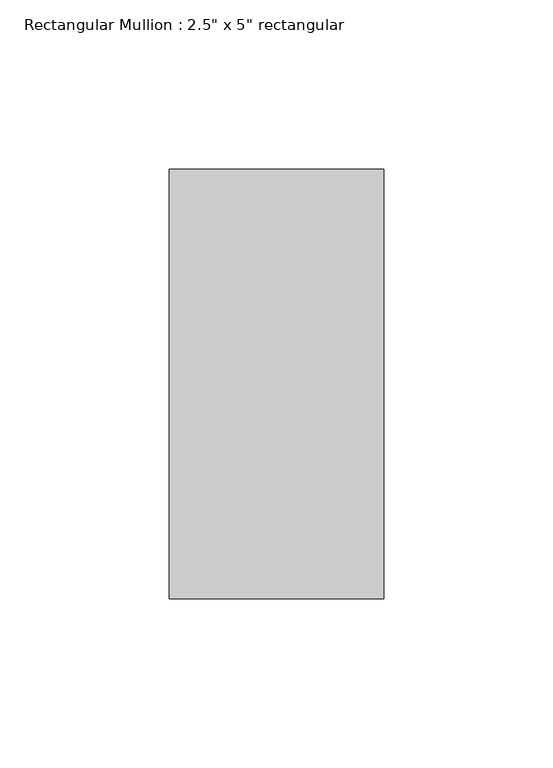
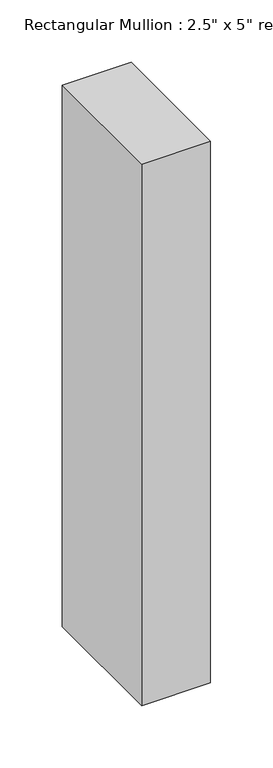
"""IFC4 building model written with IfcOpenShell, lengths in millimetres: member geometry."""

from ifc_helpers import new_model, si_unit, frame, origin, place, context, project, spatial, polyline, outline, extrude, source, transform, mapped, element, save


def member_b2ed26c7(model_context):
    return source(origin(), model_context, "Body", "SweptSolid", [
        extrude(outline(polyline([(0.0, 63.5), (0.0, -63.5), (-63.5, -63.5), (-63.5, 63.5), (0.0, 63.5)])), frame((0.0, 0.0, -529.1666667), z_axis=(0.0, 0.0, 1.0), x_axis=(1.0, 0.0, 0.0)), (0.0, 0.0, 1.0), 529.1666667),
    ])


if __name__ == "__main__":
    model = new_model("IFC4")
    model_context = context("Model", 3, world=origin())
    ifc_project = project(units=[si_unit("LENGTHUNIT", "METRE", prefix="MILLI")], contexts=[model_context])
    site = spatial("IfcSite", under=ifc_project)
    building = spatial("IfcBuilding", under=site)
    placement = place(None, origin())
    member_shape = member_b2ed26c7(model_context)
    element("IfcMember", 1, ObjectType="Rectangular Mullion : 2.5\" x 5\" rectangular", at=placement, inside=building, context=model_context, shape_type="MappedRepresentation", body=[
        mapped(member_shape, transform((0.0, 0.0, 0.0), x_axis=(1.0, 0.0, 0.0), y_axis=(0.0, 1.0, 0.0), z_axis=(0.0, 0.0, 1.0))),
    ])
    save(model, "model.ifc")

# Revit data of these elements
# Type "Rectangular Mullion : 2.5\" x 5\" rectangular"
#   built-in parameter 1007304 = 0.416667 (stored number, unit not read)
#   built-in parameter 1007301 = 0.104167 (stored number, unit not read)
#   built-in parameter 1007300 = 0.104167 (stored number, unit not read)
# Element 1 (IfcMember, "Rectangular Mullion : 2.5\" x 5\" rectangular")
#   Materials on its faces: "Aluminum"
# Materials
#   "Aluminum": class "Metal", colour RGB 247 247 247, transparency 0, Description = "Aluminum 6061", Cost = 0
